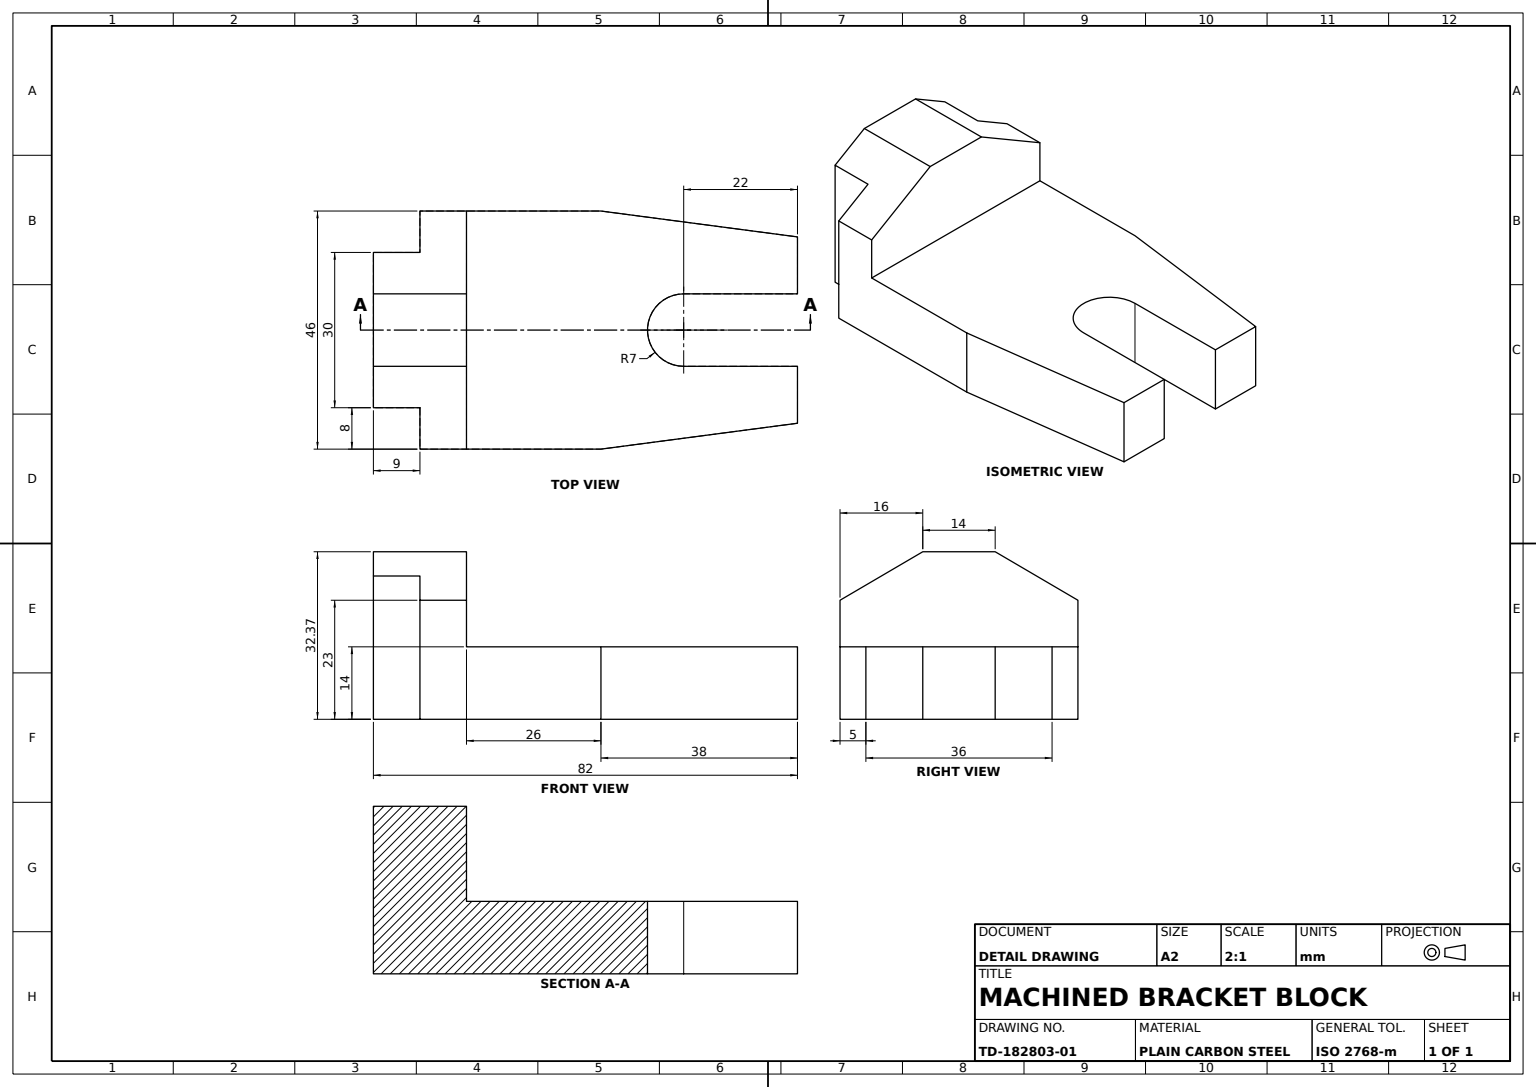
SolidWorks part; units mm, degrees
material "Plain Carbon Steel"
ref_plane "Front Plane" through (0, 0, 0) normal (0, 0, 1) x (1, 0, 0)
ref_plane "Top Plane" through (0, 0, 0) normal (0, 1, 0) x (1, 0, 0)
ref_plane "Right Plane" through (0, 0, 0) normal (1, 0, 0) x (0, 0, -1)
sketch "Slotted Base Plate Sketch" plane through (0, 0, 0) normal (0, 1, 0) x (1, 0, 0)
  line L0 (-36.5274, -13.5267) -> (-10.5274, -13.5267)
  line L1 (5.4726, 2.4733) -> (27.4726, 2.4733)
  line L2 (5.4726, 16.4733) -> (27.4726, 16.4733)
  line L3 (27.4726, 2.4733) -> (27.4726, -8.5267)
  line L6 (-36.5274, -13.5267) -> (-36.5274, 32.4733)
  line L9 (27.4726, 27.4733) -> (27.4726, 16.4733)
  line L10 (-10.5274, -13.5267) -> (27.4726, -8.5267)
  line L11 (-36.5274, 32.4733) -> (-10.5274, 32.4733)
  line L12 (-10.5274, 32.4733) -> (27.4726, 27.4733)
  line L13 (-36.5274, 32.4733) -> (-45.5274, 32.4733)
  line L14 (-45.5274, 32.4733) -> (-45.5274, 24.4733)
  line L15 (-45.5274, 24.4733) -> (-54.5274, 24.4733)
  line L16 (-54.5274, 24.4733) -> (-54.5274, -5.5267)
  line L17 (-54.5274, -5.5267) -> (-45.5274, -5.5267)
  line L18 (-45.5274, -5.5267) -> (-45.5274, -13.5267)
  line L19 (-45.5274, -13.5267) -> (-36.5274, -13.5267)
  arc A0 (5.4726, 16.4733) -> (5.4726, 2.4733) centre (5.4726, 9.4733) ccw
  dimension "D3" = 14
  dimension "D1" = 46
  dimension "D2" = 11
  dimension "D4" = 11
  dimension "D5" = 14
  dimension "D6" = 26
  dimension "D7" = 38
  dimension "D8" = 38
  dimension "D9" = 26
  dimension "D10" = 9
  dimension "D11" = 8
  dimension "D12" = 30
  dimension "D13" = 9
  dimension "D14" = 8
  dimension "D15" = 9
  dimension "D16" = 9
  dimension "D17" = 22
  dimension "D18" = 36.5274
  dimension "D19" = 13.5267
extrude "Slotted Base Plate" add sketch "Slotted Base Plate Sketch" along normal blind 14 contours L18 L19 L6 L13 L14 L15 L16 L17 | A0 L2 L9 L12 L11 L6 L0 L10 L3 L1
sketch "Rear Upright Block Sketch" plane through (0, 0, 0) normal (0, 1, 0) x (1, 0, 0)
  line L0 (-45.5274, 32.4733) -> (-36.5274, 32.4733)
  line L1 (-10.5274, 32.4733) -> (-45.5274, 32.4733) construction
  line L2 (-36.5274, 32.4733) -> (-36.5274, -13.5267)
  line L3 (-45.5274, -13.5267) -> (-10.5274, -13.5267) construction
  line L4 (-36.5274, -13.5267) -> (-45.5274, -13.5267)
  line L5 (-45.5274, -13.5267) -> (-45.5274, -5.5267)
  line L6 (-45.5274, -5.5267) -> (-54.5274, -5.5267)
  line L7 (-54.5274, -5.5267) -> (-54.5274, 24.4733)
  line L8 (-54.5274, 24.4733) -> (-45.5274, 24.4733)
  line L9 (-45.5274, 24.4733) -> (-45.5274, 32.4733)
  dimension "D1" = 9
  dimension "D2" = 9
extrude "Rear Upright Block" add sketch "Rear Upright Block Sketch" along normal blind 23
sketch "Upper Step Sketch" plane through (-36.5274, 0, 0) normal (1, 0, 0) x (0, 0, -1)
  line L0 (-13.5267, 23) -> (32.4733, 23)
  line L3 (16.4733, 32.3687) -> (2.4733, 32.3687)
  line L4 (2.4733, 32.3687) -> (-13.5267, 23)
  line L5 (32.4733, 14) -> (-13.5267, 14) construction
  line L6 (16.4733, 32.3687) -> (32.4733, 23)
  point P9 (9.4733, 32.3687)
  dimension "D1" = 7
  dimension "D2" = 14
  dimension "D3" = 16
  dimension "D4" = 18.3687
extrude "Upper Step Block" add sketch "Upper Step Sketch" against normal blind 9
sketch "Top Block Sketch" plane through (-45.5274, 0, 0) normal (-1, 0, 0) x (0, 0, 1)
  line L0 (-24.4733, 23) -> (-24.4733, 27.6844)
  line L1 (-32.4733, 23) -> (-16.4733, 32.3687) construction
  line L2 (-24.4733, 27.6844) -> (-16.4733, 32.3687)
  line L3 (-16.4733, 32.3687) -> (-2.4733, 32.3687)
  line L4 (-16.4733, 32.3687) -> (-2.4733, 32.3687) construction
  line L5 (-2.4733, 32.3687) -> (5.5267, 27.6844)
  line L6 (-2.4733, 32.3687) -> (13.5267, 23) construction
  line L7 (5.5267, 27.6844) -> (5.5267, 23)
  line L8 (5.5267, 23) -> (-24.4733, 23)
extrude "Top Block" add sketch "Top Block Sketch" along normal blind 9
